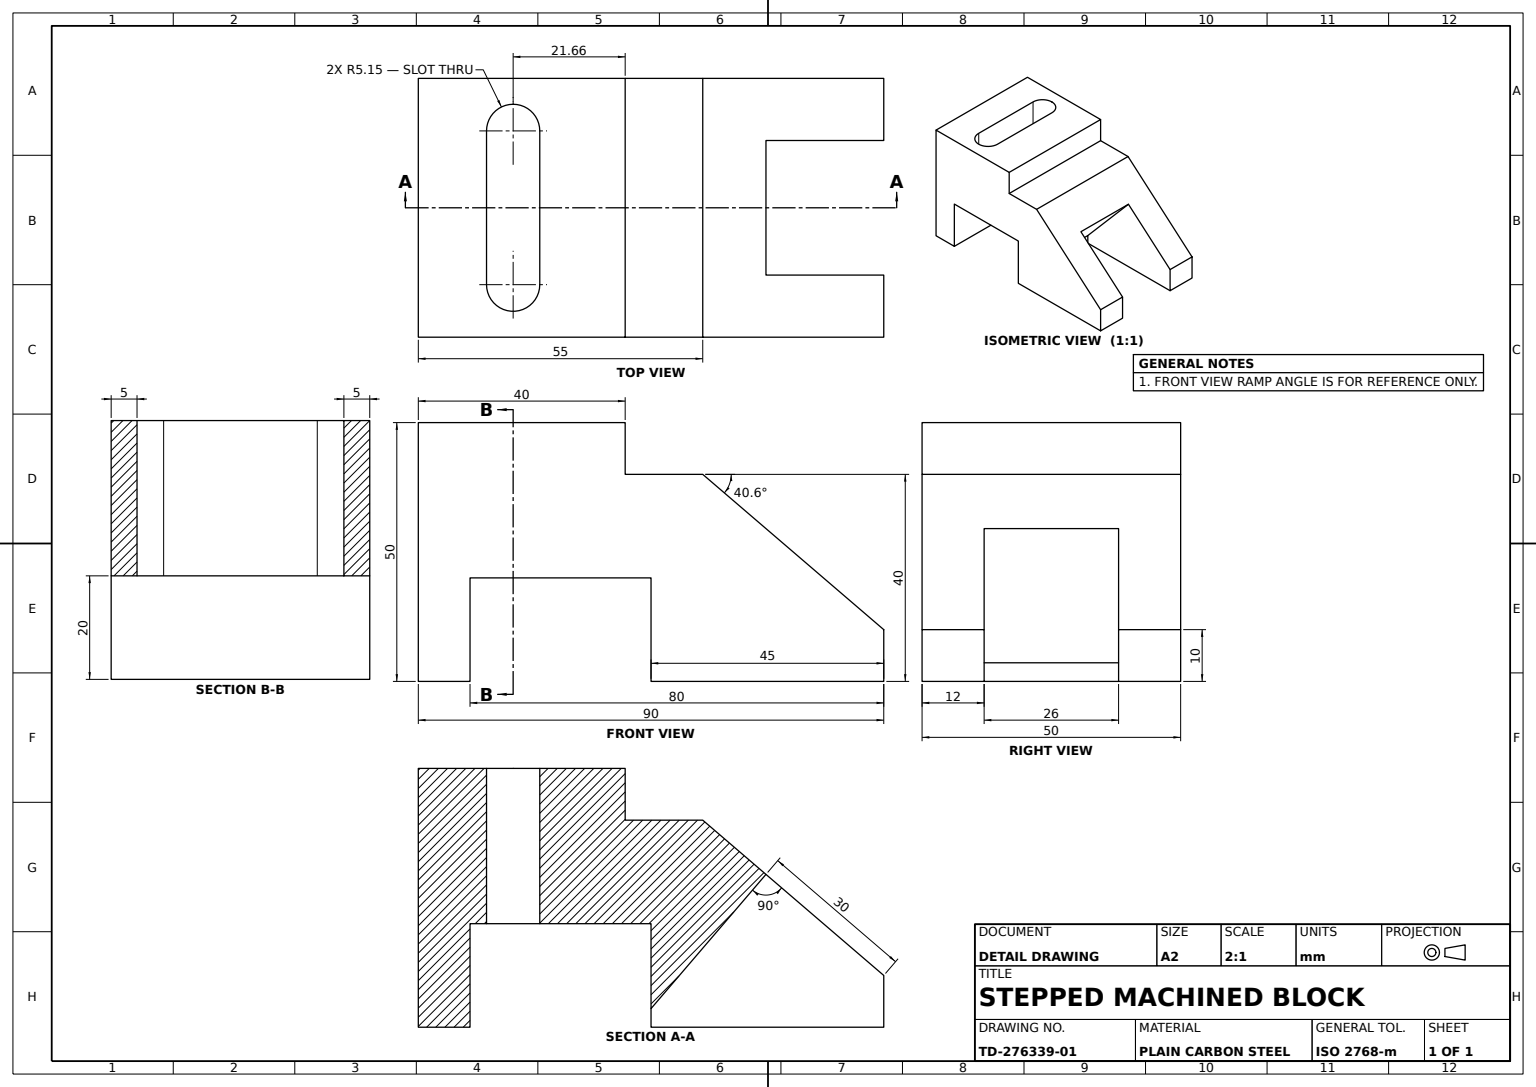
from build123d import *

# Parameters (mm, degrees)
SUPPORT_BODY_50MM_DEPTH    = 50
TOP_SLOT_34MM_DEEP_DEPTH   = 34
CLEVIS_NOTCH_SKETCH_W      = 30
CLEVIS_NOTCH_SKETCH_H      = 26
CLEVIS_NOTCH_DEPTH         = 117.062863291
SIDE_RELIEF_SKETCH_W       = 26
SIDE_RELIEF_SKETCH_H       = 10
SIDE_RELIEF_CUT_10MM_DEPTH = 10


with BuildPart() as part:
    # Support Profile Sketch → Support Body 50mm (new body)
    with BuildSketch(Plane.XY):
        Polygon((0, 0), (45, 0), (45, 20), (80, 20), (80, 0), (90, 0), (90, 50), (50, 50), (50, 40), (35, 40), (0, 10), align=None)
    extrude(amount=SUPPORT_BODY_50MM_DEPTH)

    # Top Slot Sketch → Top Slot 34mm Deep (cut)
    with BuildSketch(Plane(origin=(0, 50, 0), x_dir=(1, 0, 0), z_dir=(0, 1, 0))):
        with BuildLine():
            Line((76.808802697, -10.147055453), (76.808802697, -39.852944547))
            ThreePointArc((76.808802697, -39.852944547), (71.661747244, -45), (66.514691792, -39.852944547))
            Line((66.514691792, -39.852944547), (66.514691792, -10.147055453))
            ThreePointArc((66.514691792, -10.147055453), (71.661747244, -5), (76.808802697, -10.147055453))
        make_face()
    extrude(amount=-TOP_SLOT_34MM_DEEP_DEPTH, mode=Mode.SUBTRACT)

    # Clevis Notch Sketch → Clevis Notch (cut, through all)
    with BuildSketch(Plane(origin=(-4.941176471, 5.764705882, 0), x_dir=(0.7592566023652966, 0.6507913734559686, 0), z_dir=(-0.6507913734559686, 0.7592566023652966, 0))):
        with Locations((21.507913735, -25)):
            Rectangle(CLEVIS_NOTCH_SKETCH_W, CLEVIS_NOTCH_SKETCH_H)
    extrude(amount=-CLEVIS_NOTCH_DEPTH, mode=Mode.SUBTRACT)

    # Side Relief Sketch → Side Relief Cut 10mm (cut)
    with BuildSketch(Plane.ZY):
        with Locations((25, 5)):
            Rectangle(SIDE_RELIEF_SKETCH_W, SIDE_RELIEF_SKETCH_H)
    extrude(amount=-SIDE_RELIEF_CUT_10MM_DEPTH, mode=Mode.SUBTRACT)


solid = part.part
